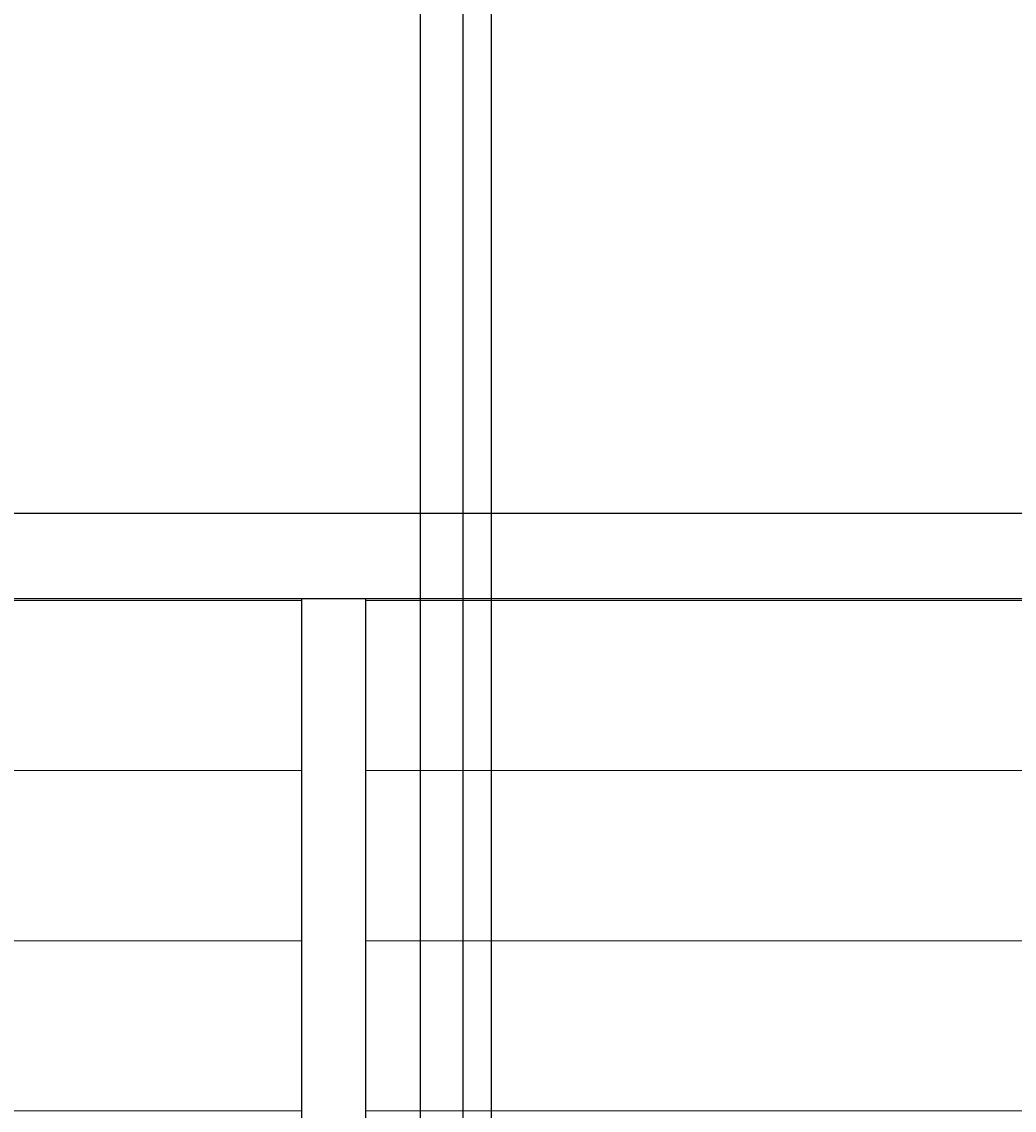
# Model space of a CAD drawing. Units: inches. Extents: x -6 to 289, y -8 to 323.
# Tile 32 of 107: x 174 to 209, y 30 to 68. Entities that reach past the tile are written whole.
import ezdxf

# ---------------------------------------------------------------- set-up
doc = ezdxf.new("R2010")
doc.units = ezdxf.units.IN
doc.header["$MEASUREMENT"] = 0
for name, color, linetype, lineweight in [('A-ANNO-DIMS', 2, 'Continuous', 18), ('A-DOOR', 3, 'Continuous', 25), ('A-ELEV-PATT', 8, 'Continuous', 13)]:
    doc.layers.add(name, color=color, linetype=linetype, lineweight=lineweight)
doc.styles.get("Standard").update_dxf_attribs({"font": 'arial.ttf'})
doc.dimstyles.get("Standard").update_dxf_attribs({"dimtxt": 0.18, "dimasz": 0.18, "dimexe": 0.18, "dimexo": 0.0625, "dimgap": 0.09, "dimtad": 0, "dimtih": 1, "dimtoh": 1, "dimdec": 4, "dimzin": 0, "dimdsep": 46, "dimtxsty": 'Standard', "dimcen": 0.09, "dimadec": 0, "dimazin": 0, "dimtfac": 1, "dimtdec": 4, "dimtofl": 0, "dimtmove": 0, "dimatfit": 3, "dimfxl": 1, "dimtolj": 1, "dimtzin": 0, "dimarcsym": 0})

# ---------------------------------------------------------------- blocks, each defined once
blk = doc.blocks.new('*D16')
at = {"layer": 'A-ANNO-DIMS', "color": 0, "lineweight": -2, "transparency": 16777216}
for p, q in [((9.943, 68.37), (9.943, -8.391)), ((272.973, 68.37), (272.973, -8.391)), ((10.123, -8.211), (140.993, -8.211)), ((272.793, -8.211), (141.923, -8.211))]:
    blk.add_line(p, q, dxfattribs=at)
at = {"layer": 'A-ANNO-DIMS', "color": 0, "transparency": 16777216}
for points in [[(10.123, -8.181), (10.123, -8.241), (9.943, -8.211)], [(272.793, -8.181), (272.793, -8.241), (272.973, -8.211)]]:
    blk.add_solid(points, dxfattribs=at)
at = {"layer": 'Defpoints', "color": 0, "transparency": 16777216}
for p in [(9.943, 68.432), (272.973, 68.432), (272.973, -8.211)]:
    blk.add_point(p, dxfattribs=at)
at = {"layer": 'A-ANNO-DIMS', "color": 0, "transparency": 16777216, "insert": (141.458, -8.211), "char_height": 0.18, "attachment_point": 5}
blk.add_mtext('\\A1;263.03', dxfattribs=at)
blk = doc.blocks.new('*D40')
at = {"layer": 'A-ANNO-DIMS', "color": 0, "lineweight": -2, "transparency": 16777216}
for p, q in [((188.292, 226.826), (188.292, -8.391)), ((189.792, 225.326), (189.792, -8.391)), ((188.472, -8.211), (188.796, -8.211)), ((189.612, -8.211), (189.288, -8.211))]:
    blk.add_line(p, q, dxfattribs=at)
at = {"layer": 'A-ANNO-DIMS', "color": 0, "transparency": 16777216}
for points in [[(188.472, -8.181), (188.472, -8.241), (188.292, -8.211)], [(189.612, -8.181), (189.612, -8.241), (189.792, -8.211)]]:
    blk.add_solid(points, dxfattribs=at)
at = {"layer": 'Defpoints', "color": 0, "transparency": 16777216}
for p in [(188.292, 226.889), (189.792, 225.389), (189.792, -8.211)]:
    blk.add_point(p, dxfattribs=at)
at = {"layer": 'A-ANNO-DIMS', "color": 0, "transparency": 16777216, "insert": (189.042, -8.211), "char_height": 0.18, "attachment_point": 5}
blk.add_mtext('\\A1;1.5', dxfattribs=at)
blk = doc.blocks.new('*D41')
at = {"layer": 'A-ANNO-DIMS', "color": 0, "lineweight": -2, "transparency": 16777216}
for p, q in [((189.792, 225.326), (189.792, -8.391)), ((190.792, 224.326), (190.792, -8.391)), ((189.972, -8.211), (190.169, -8.211)), ((190.612, -8.211), (190.415, -8.211))]:
    blk.add_line(p, q, dxfattribs=at)
at = {"layer": 'A-ANNO-DIMS', "color": 0, "transparency": 16777216}
for points in [[(189.972, -8.181), (189.972, -8.241), (189.792, -8.211)], [(190.612, -8.181), (190.612, -8.241), (190.792, -8.211)]]:
    blk.add_solid(points, dxfattribs=at)
at = {"layer": 'Defpoints', "color": 0, "transparency": 16777216}
for p in [(189.792, 225.389), (190.792, 224.389), (190.792, -8.211)]:
    blk.add_point(p, dxfattribs=at)
at = {"layer": 'A-ANNO-DIMS', "color": 0, "transparency": 16777216, "insert": (190.292, -8.211), "char_height": 0.18, "attachment_point": 5}
blk.add_mtext('\\A1;1', dxfattribs=at)
blk = doc.blocks.new('*D42')
at = {"layer": 'A-ANNO-DIMS', "color": 0, "lineweight": -2, "transparency": 16777216}
for p, q in [((190.792, 224.326), (190.792, -8.391)), ((211.292, 224.326), (211.292, -8.391)), ((190.972, -8.211), (200.716, -8.211)), ((211.112, -8.211), (201.368, -8.211))]:
    blk.add_line(p, q, dxfattribs=at)
at = {"layer": 'A-ANNO-DIMS', "color": 0, "transparency": 16777216}
for points in [[(190.972, -8.181), (190.972, -8.241), (190.792, -8.211)], [(211.112, -8.181), (211.112, -8.241), (211.292, -8.211)]]:
    blk.add_solid(points, dxfattribs=at)
at = {"layer": 'Defpoints', "color": 0, "transparency": 16777216}
for p in [(190.792, 224.389), (211.292, 224.389), (211.292, -8.211)]:
    blk.add_point(p, dxfattribs=at)
at = {"layer": 'A-ANNO-DIMS', "color": 0, "transparency": 16777216, "insert": (201.042, -8.211), "char_height": 0.18, "attachment_point": 5}
blk.add_mtext('\\A1;20.5', dxfattribs=at)

msp = doc.modelspace()

# ---------------------------------------------------------------- hatches: boundary and pattern name
at = {"layer": 'A-ELEV-PATT'}
h = msp.add_hatch(dxfattribs=at)
h.set_pattern_fill('_USER', color=256, scale=6, pattern_type=0)
h.set_pattern_definition([(0, (0, 0), (0, 6), [])])
h.paths.add_polyline_path([(184.1244, 48.0851), (124.008, 48.0851), (124.008, 10.2888), (184.1244, 10.2888)])
h.paths.add_polyline_path([(244.2408, 48.0851), (186.3604, 48.0851), (186.3604, 10.2888), (244.2408, 10.2888)])
h.paths.add_polyline_path([(208.2918, 114.2795), (190.7918, 114.2795), (190.7918, 71.2795), (208.2918, 71.2795)])
h.paths.add_polyline_path([(227.7918, 114.2795), (209.2918, 114.2795), (209.2918, 71.2795), (227.7918, 71.2795)])
h.paths.add_polyline_path([(211.2918, 224.3887), (190.7918, 224.3887), (190.7918, 162.3484), (211.2918, 162.3484)])
h.paths.add_polyline_path([(233.7918, 224.3887), (212.2918, 224.3887), (212.2918, 162.3484), (233.7918, 162.3484)])
h.paths.add_polyline_path([(166.3835, 224.154), (147.8835, 224.154), (147.8835, 181.154), (166.3835, 181.154)])
h.paths.add_polyline_path([(146.8835, 224.154), (129.3835, 224.154), (129.3835, 181.154), (146.8835, 181.154)])

# ---------------------------------------------------------------- linework, layer by layer
at = {"layer": 'A-DOOR'}
for points in [[(121.008, 51.0851), (247.2408, 51.0851), (247.2408, 7.2888), (121.008, 7.2888)], [(124.008, 48.0851), (244.2408, 48.0851), (244.2408, 10.2888), (124.008, 10.2888)], [(184.1244, 48.0851), (186.3604, 48.0851), (186.3604, 10.2888), (184.1244, 10.2888)]]:
    msp.add_lwpolyline(points, close=True, dxfattribs=at)

# ---------------------------------------------------------------- dimensions: what is measured, and where the dimension line sits
at = {"layer": 'A-ANNO-DIMS'}
for base, p1, p2, override, picture, middle in [((189.7918, -8.2112), (188.2918, 226.8887), (189.7918, 225.3887), {"dimdec": 1, "dimlfac": 1, "dimrnd": 0, "dimzin": 0, "dimdsep": 46, "dimlunit": 2}, '*D40', (189.0418, -8.2112)), ((190.7918, -8.2112), (189.7918, 225.3887), (190.7918, 224.3887), {"dimdec": 0, "dimlfac": 1, "dimrnd": 0, "dimzin": 0, "dimdsep": 46, "dimlunit": 2}, '*D41', (190.2918, -8.2112)), ((211.2918, -8.2112), (190.7918, 224.3887), (211.2918, 224.3887), {"dimdec": 1, "dimlfac": 1, "dimrnd": 0, "dimzin": 0, "dimdsep": 46, "dimlunit": 2}, '*D42', (201.0418, -8.2112)), ((272.9733, -8.2112), (9.943, 68.4322), (272.9733, 68.4322), {"dimdec": 2, "dimlfac": 1, "dimrnd": 0, "dimzin": 0, "dimdsep": 46, "dimlunit": 2}, '*D16', (141.4581, -8.2112))]:
    dim = msp.add_linear_dim(base=base, p1=p1, p2=p2, dimstyle='Standard', override=override, dxfattribs=at)
    dim.commit()
    dim.dimension.update_dxf_attribs({"geometry": picture, "text_midpoint": middle})

doc.saveas('drawing.dxf')
